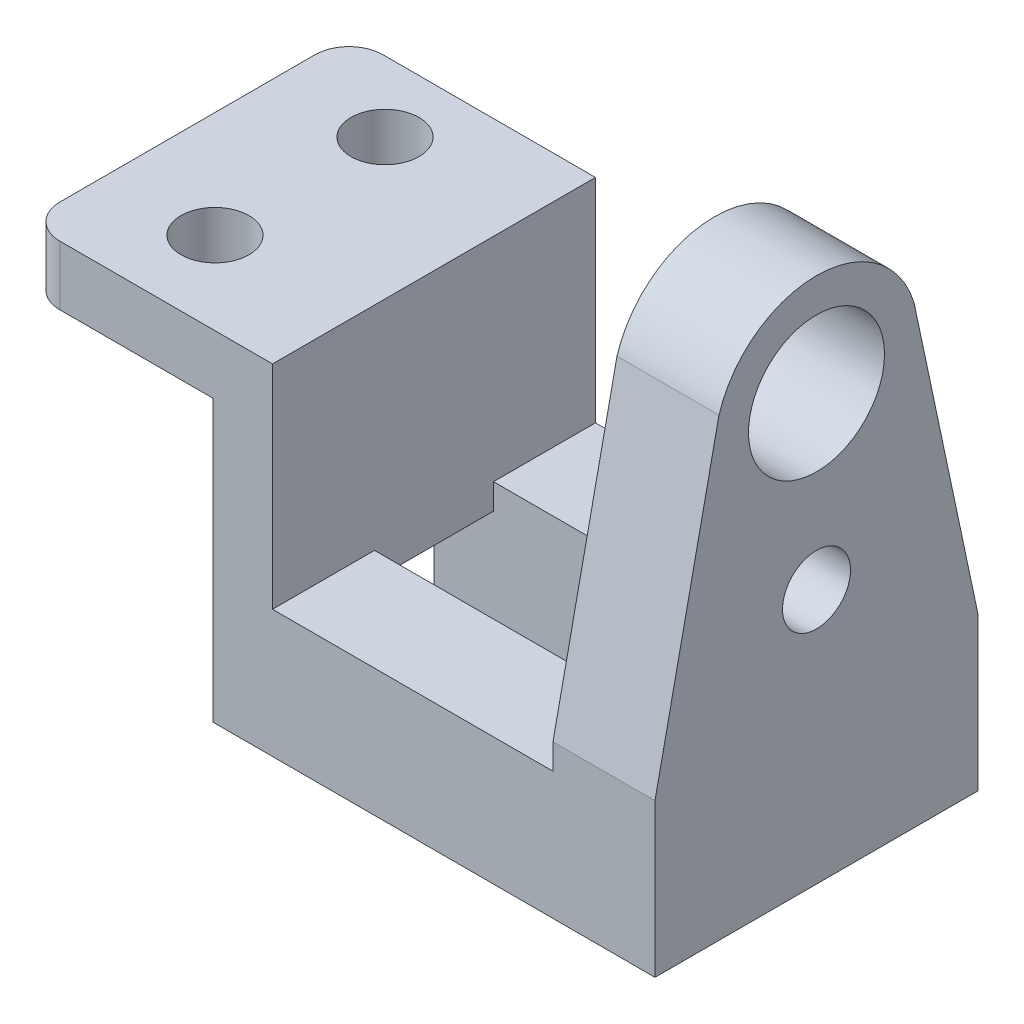
ISO-10303-21;
HEADER;
FILE_DESCRIPTION(('STEP AP214'),'2;1');
FILE_NAME('part.step','',(''),(''),'','','');
FILE_SCHEMA(('AUTOMOTIVE_DESIGN { 1 0 10303 214 1 1 1 1 }'));
ENDSEC;
DATA;
#1=APPLICATION_CONTEXT('core data for automotive mechanical design processes');
#2=APPLICATION_PROTOCOL_DEFINITION('international standard','automotive_design',2000,#1);
#3=PRODUCT_CONTEXT('',#1,'mechanical');
#4=PRODUCT('Part','Part','',(#3));
#5=PRODUCT_RELATED_PRODUCT_CATEGORY('part','',(#4));
#6=PRODUCT_DEFINITION_FORMATION('','',#4);
#7=PRODUCT_DEFINITION_CONTEXT('part definition',#1,'design');
#8=PRODUCT_DEFINITION('design','',#6,#7);
#9=PRODUCT_DEFINITION_SHAPE('','',#8);
#10=(LENGTH_UNIT() NAMED_UNIT(*) SI_UNIT(.MILLI.,.METRE.));
#11=(NAMED_UNIT(*) PLANE_ANGLE_UNIT() SI_UNIT($,.RADIAN.));
#12=(NAMED_UNIT(*) SI_UNIT($,.STERADIAN.) SOLID_ANGLE_UNIT());
#13=UNCERTAINTY_MEASURE_WITH_UNIT(LENGTH_MEASURE(1.E-05),#10,'distance_accuracy_value','');
#14=(GEOMETRIC_REPRESENTATION_CONTEXT(3) GLOBAL_UNCERTAINTY_ASSIGNED_CONTEXT((#13)) GLOBAL_UNIT_ASSIGNED_CONTEXT((#10,
#11,#12)) REPRESENTATION_CONTEXT('',''));
#15=CARTESIAN_POINT('',(0.,0.,0.));
#16=DIRECTION('',(0.,0.,1.));
#17=DIRECTION('',(1.,0.,0.));
#18=AXIS2_PLACEMENT_3D('',#15,#16,#17);
#19=CARTESIAN_POINT('',(7.,8.,38.));
#20=DIRECTION('',(-1.,0.,0.));
#21=DIRECTION('',(0.,0.,1.));
#22=AXIS2_PLACEMENT_3D('',#19,#20,#21);
#23=PLANE('',#22);
#24=DIRECTION('',(0.,-1.,0.));
#25=VECTOR('',#24,1.);
#26=CARTESIAN_POINT('',(7.,15.,12.));
#27=LINE('',#26,#25);
#28=CARTESIAN_POINT('',(7.,15.,12.));
#29=VERTEX_POINT('',#28);
#30=CARTESIAN_POINT('',(6.99999999999998,12.,12.));
#31=VERTEX_POINT('',#30);
#32=EDGE_CURVE('E58',#29,#31,#27,.T.);
#33=ORIENTED_EDGE('',*,*,#32,.F.);
#34=DIRECTION('',(0.,0.,1.));
#35=VECTOR('',#34,1.);
#36=CARTESIAN_POINT('',(7.,15.,12.));
#37=LINE('',#36,#35);
#38=CARTESIAN_POINT('',(7.,15.,0.));
#39=VERTEX_POINT('',#38);
#40=EDGE_CURVE('E406',#39,#29,#37,.T.);
#41=ORIENTED_EDGE('',*,*,#40,.F.);
#42=DIRECTION('',(0.,1.,0.));
#43=VECTOR('',#42,1.);
#44=CARTESIAN_POINT('',(7.,8.,0.));
#45=LINE('',#44,#43);
#46=CARTESIAN_POINT('',(7.,40.,0.));
#47=VERTEX_POINT('',#46);
#48=EDGE_CURVE('E292',#39,#47,#45,.T.);
#49=ORIENTED_EDGE('',*,*,#48,.T.);
#50=DIRECTION('',(0.,0.,1.));
#51=VECTOR('',#50,1.);
#52=CARTESIAN_POINT('',(7.,40.,0.));
#53=LINE('',#52,#51);
#54=CARTESIAN_POINT('',(7.,40.,38.));
#55=VERTEX_POINT('',#54);
#56=EDGE_CURVE('E236',#47,#55,#53,.T.);
#57=ORIENTED_EDGE('',*,*,#56,.T.);
#58=DIRECTION('',(0.,1.,0.));
#59=VECTOR('',#58,1.);
#60=CARTESIAN_POINT('',(7.,8.,38.));
#61=LINE('',#60,#59);
#62=CARTESIAN_POINT('',(7.,15.,38.));
#63=VERTEX_POINT('',#62);
#64=EDGE_CURVE('E301',#63,#55,#61,.T.);
#65=ORIENTED_EDGE('',*,*,#64,.F.);
#66=DIRECTION('',(0.,0.,1.));
#67=VECTOR('',#66,1.);
#68=CARTESIAN_POINT('',(7.,15.,38.));
#69=LINE('',#68,#67);
#70=CARTESIAN_POINT('',(7.,15.,26.));
#71=VERTEX_POINT('',#70);
#72=EDGE_CURVE('E349',#71,#63,#69,.T.);
#73=ORIENTED_EDGE('',*,*,#72,.F.);
#74=DIRECTION('',(0.,-1.,0.));
#75=VECTOR('',#74,1.);
#76=CARTESIAN_POINT('',(7.,15.,26.));
#77=LINE('',#76,#75);
#78=CARTESIAN_POINT('',(7.,12.,26.));
#79=VERTEX_POINT('',#78);
#80=EDGE_CURVE('E348',#71,#79,#77,.T.);
#81=ORIENTED_EDGE('',*,*,#80,.T.);
#82=DIRECTION('',(0.,0.,1.));
#83=VECTOR('',#82,1.);
#84=CARTESIAN_POINT('',(7.,12.,38.));
#85=LINE('',#84,#83);
#86=EDGE_CURVE('E11',#31,#79,#85,.T.);
#87=ORIENTED_EDGE('',*,*,#86,.F.);
#88=EDGE_LOOP('',(#33,#41,#49,#57,#65,#73,#81,#87));
#89=FACE_BOUND('',#88,.T.);
#90=ADVANCED_FACE('F44',(#89),#23,.F.);
#91=CARTESIAN_POINT('',(40.,18.,38.));
#92=DIRECTION('',(1.,0.,0.));
#93=DIRECTION('',(0.,0.,-1.));
#94=AXIS2_PLACEMENT_3D('',#91,#92,#93);
#95=PLANE('',#94);
#96=CARTESIAN_POINT('',(40.,30.,19.));
#97=DIRECTION('',(1.,0.,0.));
#98=DIRECTION('',(0.,0.,-1.));
#99=AXIS2_PLACEMENT_3D('',#96,#97,#98);
#100=CIRCLE('',#99,4.);
#101=CARTESIAN_POINT('',(40.,30.,15.));
#102=VERTEX_POINT('',#101);
#103=EDGE_CURVE('E357',#102,#102,#100,.T.);
#104=ORIENTED_EDGE('',*,*,#103,.T.);
#105=EDGE_LOOP('',(#104));
#106=FACE_BOUND('',#105,.T.);
#107=CARTESIAN_POINT('',(40.,50.,19.));
#108=DIRECTION('',(1.,0.,0.));
#109=DIRECTION('',(0.,0.,-1.));
#110=AXIS2_PLACEMENT_3D('',#107,#108,#109);
#111=CIRCLE('',#110,8.);
#112=CARTESIAN_POINT('',(40.,50.,11.));
#113=VERTEX_POINT('',#112);
#114=EDGE_CURVE('E366',#113,#113,#111,.T.);
#115=ORIENTED_EDGE('',*,*,#114,.T.);
#116=EDGE_LOOP('',(#115));
#117=FACE_BOUND('',#116,.T.);
#118=DIRECTION('',(0.,0.,-1.));
#119=VECTOR('',#118,1.);
#120=CARTESIAN_POINT('',(40.,15.,0.));
#121=LINE('',#120,#119);
#122=CARTESIAN_POINT('',(40.,15.,12.));
#123=VERTEX_POINT('',#122);
#124=CARTESIAN_POINT('',(40.,15.,0.));
#125=VERTEX_POINT('',#124);
#126=EDGE_CURVE('E410',#123,#125,#121,.T.);
#127=ORIENTED_EDGE('',*,*,#126,.F.);
#128=DIRECTION('',(0.,1.,0.));
#129=VECTOR('',#128,1.);
#130=CARTESIAN_POINT('',(40.,12.,12.));
#131=LINE('',#130,#129);
#132=CARTESIAN_POINT('',(40.,0.,12.));
#133=VERTEX_POINT('',#132);
#134=EDGE_CURVE('E70',#133,#123,#131,.T.);
#135=ORIENTED_EDGE('',*,*,#134,.F.);
#136=DIRECTION('',(0.,0.,-1.));
#137=VECTOR('',#136,1.);
#138=CARTESIAN_POINT('',(40.,0.,38.));
#139=LINE('',#138,#137);
#140=CARTESIAN_POINT('',(40.,0.,26.));
#141=VERTEX_POINT('',#140);
#142=EDGE_CURVE('E239',#141,#133,#139,.T.);
#143=ORIENTED_EDGE('',*,*,#142,.F.);
#144=DIRECTION('',(0.,-1.,0.));
#145=VECTOR('',#144,1.);
#146=CARTESIAN_POINT('',(40.,0.,26.));
#147=LINE('',#146,#145);
#148=CARTESIAN_POINT('',(40.,15.,26.));
#149=VERTEX_POINT('',#148);
#150=EDGE_CURVE('E241',#149,#141,#147,.T.);
#151=ORIENTED_EDGE('',*,*,#150,.F.);
#152=DIRECTION('',(0.,0.,-1.));
#153=VECTOR('',#152,1.);
#154=CARTESIAN_POINT('',(40.,15.,26.));
#155=LINE('',#154,#153);
#156=CARTESIAN_POINT('',(40.,15.,38.));
#157=VERTEX_POINT('',#156);
#158=EDGE_CURVE('E360',#157,#149,#155,.T.);
#159=ORIENTED_EDGE('',*,*,#158,.F.);
#160=DIRECTION('',(0.,-1.,0.));
#161=VECTOR('',#160,1.);
#162=CARTESIAN_POINT('',(40.,18.,38.));
#163=LINE('',#162,#161);
#164=CARTESIAN_POINT('',(40.,18.,38.));
#165=VERTEX_POINT('',#164);
#166=EDGE_CURVE('E296',#165,#157,#163,.T.);
#167=ORIENTED_EDGE('',*,*,#166,.F.);
#168=DIRECTION('',(0.,-0.978272196346445,0.207324648451413));
#169=VECTOR('',#168,1.);
#170=CARTESIAN_POINT('',(40.,18.,38.));
#171=LINE('',#170,#169);
#172=CARTESIAN_POINT('',(40.,53.5184745322787,30.4725906823919));
#173=VERTEX_POINT('',#172);
#174=EDGE_CURVE('E270',#173,#165,#171,.T.);
#175=ORIENTED_EDGE('',*,*,#174,.F.);
#176=CARTESIAN_POINT('',(40.,50.,19.));
#177=DIRECTION('',(1.,0.,0.));
#178=DIRECTION('',(0.,0.,-1.));
#179=AXIS2_PLACEMENT_3D('',#176,#177,#178);
#180=CIRCLE('',#179,12.);
#181=CARTESIAN_POINT('',(40.,53.5184745322787,7.52740931760806));
#182=VERTEX_POINT('',#181);
#183=EDGE_CURVE('E274',#182,#173,#180,.T.);
#184=ORIENTED_EDGE('',*,*,#183,.F.);
#185=DIRECTION('',(0.,0.978272196346445,0.207324648451413));
#186=VECTOR('',#185,1.);
#187=CARTESIAN_POINT('',(40.,18.,0.));
#188=LINE('',#187,#186);
#189=CARTESIAN_POINT('',(40.,18.,0.));
#190=VERTEX_POINT('',#189);
#191=EDGE_CURVE('E267',#190,#182,#188,.T.);
#192=ORIENTED_EDGE('',*,*,#191,.F.);
#193=DIRECTION('',(0.,-1.,0.));
#194=VECTOR('',#193,1.);
#195=CARTESIAN_POINT('',(40.,18.,0.));
#196=LINE('',#195,#194);
#197=EDGE_CURVE('E315',#190,#125,#196,.T.);
#198=ORIENTED_EDGE('',*,*,#197,.T.);
#199=EDGE_LOOP('',(#127,#135,#143,#151,#159,#167,#175,#184,#192,#198));
#200=FACE_BOUND('',#199,.T.);
#201=ADVANCED_FACE('F421',(#106,#117,#200),#95,.F.);
#202=CARTESIAN_POINT('',(0.,0.,38.));
#203=DIRECTION('',(1.,0.,0.));
#204=DIRECTION('',(0.,0.,-1.));
#205=AXIS2_PLACEMENT_3D('',#202,#203,#204);
#206=PLANE('',#205);
#207=DIRECTION('',(0.,-1.,0.));
#208=VECTOR('',#207,1.);
#209=CARTESIAN_POINT('',(0.,0.,38.));
#210=LINE('',#209,#208);
#211=CARTESIAN_POINT('',(0.,33.,38.));
#212=VERTEX_POINT('',#211);
#213=CARTESIAN_POINT('',(0.,0.,38.));
#214=VERTEX_POINT('',#213);
#215=EDGE_CURVE('E289',#212,#214,#210,.T.);
#216=ORIENTED_EDGE('',*,*,#215,.F.);
#217=DIRECTION('',(0.,0.,-1.));
#218=VECTOR('',#217,1.);
#219=CARTESIAN_POINT('',(0.,33.,0.));
#220=LINE('',#219,#218);
#221=CARTESIAN_POINT('',(0.,33.,0.));
#222=VERTEX_POINT('',#221);
#223=EDGE_CURVE('E219',#212,#222,#220,.T.);
#224=ORIENTED_EDGE('',*,*,#223,.T.);
#225=DIRECTION('',(0.,-1.,0.));
#226=VECTOR('',#225,1.);
#227=CARTESIAN_POINT('',(0.,0.,0.));
#228=LINE('',#227,#226);
#229=CARTESIAN_POINT('',(0.,0.,0.));
#230=VERTEX_POINT('',#229);
#231=EDGE_CURVE('E290',#222,#230,#228,.T.);
#232=ORIENTED_EDGE('',*,*,#231,.T.);
#233=DIRECTION('',(0.,0.,-1.));
#234=VECTOR('',#233,1.);
#235=CARTESIAN_POINT('',(0.,0.,38.));
#236=LINE('',#235,#234);
#237=CARTESIAN_POINT('',(0.,0.,12.));
#238=VERTEX_POINT('',#237);
#239=EDGE_CURVE('E317',#238,#230,#236,.T.);
#240=ORIENTED_EDGE('',*,*,#239,.F.);
#241=DIRECTION('',(0.,1.,0.));
#242=VECTOR('',#241,1.);
#243=CARTESIAN_POINT('',(0.,12.,12.));
#244=LINE('',#243,#242);
#245=CARTESIAN_POINT('',(0.,12.,12.));
#246=VERTEX_POINT('',#245);
#247=EDGE_CURVE('E244',#238,#246,#244,.T.);
#248=ORIENTED_EDGE('',*,*,#247,.T.);
#249=DIRECTION('',(0.,0.,1.));
#250=VECTOR('',#249,1.);
#251=CARTESIAN_POINT('',(0.,12.,26.));
#252=LINE('',#251,#250);
#253=CARTESIAN_POINT('',(0.,12.,26.));
#254=VERTEX_POINT('',#253);
#255=EDGE_CURVE('E248',#246,#254,#252,.T.);
#256=ORIENTED_EDGE('',*,*,#255,.T.);
#257=DIRECTION('',(0.,-1.,0.));
#258=VECTOR('',#257,1.);
#259=CARTESIAN_POINT('',(0.,0.,26.));
#260=LINE('',#259,#258);
#261=CARTESIAN_POINT('',(0.,0.,26.));
#262=VERTEX_POINT('',#261);
#263=EDGE_CURVE('E246',#254,#262,#260,.T.);
#264=ORIENTED_EDGE('',*,*,#263,.T.);
#265=EDGE_CURVE('E52',#214,#262,#236,.T.);
#266=ORIENTED_EDGE('',*,*,#265,.F.);
#267=EDGE_LOOP('',(#216,#224,#232,#240,#248,#256,#264,#266));
#268=FACE_BOUND('',#267,.T.);
#269=ADVANCED_FACE('F50',(#268),#206,.F.);
#270=CARTESIAN_POINT('',(0.,0.,38.));
#271=DIRECTION('',(0.,1.,0.));
#272=DIRECTION('',(0.,0.,1.));
#273=AXIS2_PLACEMENT_3D('',#270,#271,#272);
#274=PLANE('',#273);
#275=DIRECTION('',(1.,0.,0.));
#276=VECTOR('',#275,1.);
#277=CARTESIAN_POINT('',(-111.747483193135,0.,26.));
#278=LINE('',#277,#276);
#279=EDGE_CURVE('E261',#262,#141,#278,.T.);
#280=ORIENTED_EDGE('',*,*,#279,.T.);
#281=ORIENTED_EDGE('',*,*,#142,.T.);
#282=DIRECTION('',(1.,0.,0.));
#283=VECTOR('',#282,1.);
#284=CARTESIAN_POINT('',(-111.747483193135,0.,12.));
#285=LINE('',#284,#283);
#286=EDGE_CURVE('E243',#238,#133,#285,.T.);
#287=ORIENTED_EDGE('',*,*,#286,.F.);
#288=ORIENTED_EDGE('',*,*,#239,.T.);
#289=DIRECTION('',(1.,0.,0.));
#290=VECTOR('',#289,1.);
#291=CARTESIAN_POINT('',(0.,0.,0.));
#292=LINE('',#291,#290);
#293=CARTESIAN_POINT('',(52.,0.,0.));
#294=VERTEX_POINT('',#293);
#295=EDGE_CURVE('E304',#230,#294,#292,.T.);
#296=ORIENTED_EDGE('',*,*,#295,.T.);
#297=DIRECTION('',(0.,0.,-1.));
#298=VECTOR('',#297,1.);
#299=CARTESIAN_POINT('',(52.,0.,38.));
#300=LINE('',#299,#298);
#301=CARTESIAN_POINT('',(52.,0.,38.));
#302=VERTEX_POINT('',#301);
#303=EDGE_CURVE('E303',#302,#294,#300,.T.);
#304=ORIENTED_EDGE('',*,*,#303,.F.);
#305=DIRECTION('',(1.,0.,0.));
#306=VECTOR('',#305,1.);
#307=CARTESIAN_POINT('',(0.,0.,38.));
#308=LINE('',#307,#306);
#309=EDGE_CURVE('E293',#214,#302,#308,.T.);
#310=ORIENTED_EDGE('',*,*,#309,.F.);
#311=ORIENTED_EDGE('',*,*,#265,.T.);
#312=EDGE_LOOP('',(#280,#281,#287,#288,#296,#304,#310,#311));
#313=FACE_BOUND('',#312,.T.);
#314=ADVANCED_FACE('F324',(#313),#274,.F.);
#315=CARTESIAN_POINT('',(52.,0.,38.));
#316=DIRECTION('',(-1.,0.,0.));
#317=DIRECTION('',(0.,0.,1.));
#318=AXIS2_PLACEMENT_3D('',#315,#316,#317);
#319=PLANE('',#318);
#320=CARTESIAN_POINT('',(52.,30.,19.));
#321=DIRECTION('',(1.,0.,0.));
#322=DIRECTION('',(0.,0.,-1.));
#323=AXIS2_PLACEMENT_3D('',#320,#321,#322);
#324=CIRCLE('',#323,4.);
#325=CARTESIAN_POINT('',(52.,30.,15.));
#326=VERTEX_POINT('',#325);
#327=EDGE_CURVE('E351',#326,#326,#324,.T.);
#328=ORIENTED_EDGE('',*,*,#327,.F.);
#329=EDGE_LOOP('',(#328));
#330=FACE_BOUND('',#329,.T.);
#331=CARTESIAN_POINT('',(52.,50.,19.));
#332=DIRECTION('',(1.,0.,0.));
#333=DIRECTION('',(0.,0.,-1.));
#334=AXIS2_PLACEMENT_3D('',#331,#332,#333);
#335=CIRCLE('',#334,8.);
#336=CARTESIAN_POINT('',(52.,50.,11.));
#337=VERTEX_POINT('',#336);
#338=EDGE_CURVE('E364',#337,#337,#335,.T.);
#339=ORIENTED_EDGE('',*,*,#338,.F.);
#340=EDGE_LOOP('',(#339));
#341=FACE_BOUND('',#340,.T.);
#342=DIRECTION('',(0.,1.,0.));
#343=VECTOR('',#342,1.);
#344=CARTESIAN_POINT('',(52.,0.,0.));
#345=LINE('',#344,#343);
#346=CARTESIAN_POINT('',(52.,18.,0.));
#347=VERTEX_POINT('',#346);
#348=EDGE_CURVE('E310',#294,#347,#345,.T.);
#349=ORIENTED_EDGE('',*,*,#348,.T.);
#350=DIRECTION('',(0.,0.978272196346445,0.207324648451413));
#351=VECTOR('',#350,1.);
#352=CARTESIAN_POINT('',(52.,18.,0.));
#353=LINE('',#352,#351);
#354=CARTESIAN_POINT('',(52.,53.5184745322787,7.52740931760806));
#355=VERTEX_POINT('',#354);
#356=EDGE_CURVE('E279',#347,#355,#353,.T.);
#357=ORIENTED_EDGE('',*,*,#356,.T.);
#358=CARTESIAN_POINT('',(52.,50.,19.));
#359=DIRECTION('',(1.,0.,0.));
#360=DIRECTION('',(0.,0.,-1.));
#361=AXIS2_PLACEMENT_3D('',#358,#359,#360);
#362=CIRCLE('',#361,12.);
#363=CARTESIAN_POINT('',(52.,53.5184745322787,30.4725906823919));
#364=VERTEX_POINT('',#363);
#365=EDGE_CURVE('E272',#355,#364,#362,.T.);
#366=ORIENTED_EDGE('',*,*,#365,.T.);
#367=DIRECTION('',(0.,-0.978272196346445,0.207324648451413));
#368=VECTOR('',#367,1.);
#369=CARTESIAN_POINT('',(52.,18.,38.));
#370=LINE('',#369,#368);
#371=CARTESIAN_POINT('',(52.,18.,38.));
#372=VERTEX_POINT('',#371);
#373=EDGE_CURVE('E262',#364,#372,#370,.T.);
#374=ORIENTED_EDGE('',*,*,#373,.T.);
#375=DIRECTION('',(0.,1.,0.));
#376=VECTOR('',#375,1.);
#377=CARTESIAN_POINT('',(52.,0.,38.));
#378=LINE('',#377,#376);
#379=EDGE_CURVE('E295',#302,#372,#378,.T.);
#380=ORIENTED_EDGE('',*,*,#379,.F.);
#381=ORIENTED_EDGE('',*,*,#303,.T.);
#382=EDGE_LOOP('',(#349,#357,#366,#374,#380,#381));
#383=FACE_BOUND('',#382,.T.);
#384=ADVANCED_FACE('F337',(#330,#341,#383),#319,.F.);
#385=CARTESIAN_POINT('',(0.,0.,38.));
#386=DIRECTION('',(0.,0.,1.));
#387=DIRECTION('',(1.,0.,0.));
#388=AXIS2_PLACEMENT_3D('',#385,#386,#387);
#389=PLANE('',#388);
#390=DIRECTION('',(1.,0.,0.));
#391=VECTOR('',#390,1.);
#392=CARTESIAN_POINT('',(40.,15.,38.));
#393=LINE('',#392,#391);
#394=EDGE_CURVE('E414',#63,#157,#393,.T.);
#395=ORIENTED_EDGE('',*,*,#394,.F.);
#396=ORIENTED_EDGE('',*,*,#64,.T.);
#397=DIRECTION('',(-1.,0.,0.));
#398=VECTOR('',#397,1.);
#399=CARTESIAN_POINT('',(7.,40.,38.));
#400=LINE('',#399,#398);
#401=CARTESIAN_POINT('',(-18.,40.,38.));
#402=VERTEX_POINT('',#401);
#403=EDGE_CURVE('E230',#55,#402,#400,.T.);
#404=ORIENTED_EDGE('',*,*,#403,.T.);
#405=DIRECTION('',(0.,1.,0.));
#406=VECTOR('',#405,1.);
#407=CARTESIAN_POINT('',(-18.,33.,38.));
#408=LINE('',#407,#406);
#409=CARTESIAN_POINT('',(-18.,33.,38.));
#410=VERTEX_POINT('',#409);
#411=EDGE_CURVE('E229',#410,#402,#408,.T.);
#412=ORIENTED_EDGE('',*,*,#411,.F.);
#413=DIRECTION('',(1.,0.,0.));
#414=VECTOR('',#413,1.);
#415=CARTESIAN_POINT('',(-18.,33.,38.));
#416=LINE('',#415,#414);
#417=EDGE_CURVE('E220',#410,#212,#416,.T.);
#418=ORIENTED_EDGE('',*,*,#417,.T.);
#419=ORIENTED_EDGE('',*,*,#215,.T.);
#420=ORIENTED_EDGE('',*,*,#309,.T.);
#421=ORIENTED_EDGE('',*,*,#379,.T.);
#422=DIRECTION('',(-1.,0.,0.));
#423=VECTOR('',#422,1.);
#424=CARTESIAN_POINT('',(52.,18.,38.));
#425=LINE('',#424,#423);
#426=EDGE_CURVE('E298',#372,#165,#425,.T.);
#427=ORIENTED_EDGE('',*,*,#426,.T.);
#428=ORIENTED_EDGE('',*,*,#166,.T.);
#429=EDGE_LOOP('',(#395,#396,#404,#412,#418,#419,#420,#421,#427,#428));
#430=FACE_BOUND('',#429,.T.);
#431=ADVANCED_FACE('F394',(#430),#389,.T.);
#432=CARTESIAN_POINT('',(0.,0.,0.));
#433=DIRECTION('',(0.,0.,1.));
#434=DIRECTION('',(1.,0.,0.));
#435=AXIS2_PLACEMENT_3D('',#432,#433,#434);
#436=PLANE('',#435);
#437=ORIENTED_EDGE('',*,*,#48,.F.);
#438=DIRECTION('',(-1.,0.,0.));
#439=VECTOR('',#438,1.);
#440=CARTESIAN_POINT('',(7.,15.,0.));
#441=LINE('',#440,#439);
#442=EDGE_CURVE('E397',#125,#39,#441,.T.);
#443=ORIENTED_EDGE('',*,*,#442,.F.);
#444=ORIENTED_EDGE('',*,*,#197,.F.);
#445=DIRECTION('',(-1.,0.,0.));
#446=VECTOR('',#445,1.);
#447=CARTESIAN_POINT('',(52.,18.,0.));
#448=LINE('',#447,#446);
#449=EDGE_CURVE('E307',#347,#190,#448,.T.);
#450=ORIENTED_EDGE('',*,*,#449,.F.);
#451=ORIENTED_EDGE('',*,*,#348,.F.);
#452=ORIENTED_EDGE('',*,*,#295,.F.);
#453=ORIENTED_EDGE('',*,*,#231,.F.);
#454=DIRECTION('',(-1.,0.,0.));
#455=VECTOR('',#454,1.);
#456=CARTESIAN_POINT('',(0.,33.,0.));
#457=LINE('',#456,#455);
#458=CARTESIAN_POINT('',(-18.,33.,0.));
#459=VERTEX_POINT('',#458);
#460=EDGE_CURVE('E192',#222,#459,#457,.T.);
#461=ORIENTED_EDGE('',*,*,#460,.T.);
#462=DIRECTION('',(0.,1.,0.));
#463=VECTOR('',#462,1.);
#464=CARTESIAN_POINT('',(-18.,33.,0.));
#465=LINE('',#464,#463);
#466=CARTESIAN_POINT('',(-18.,40.,0.));
#467=VERTEX_POINT('',#466);
#468=EDGE_CURVE('E210',#459,#467,#465,.T.);
#469=ORIENTED_EDGE('',*,*,#468,.T.);
#470=DIRECTION('',(-1.,0.,0.));
#471=VECTOR('',#470,1.);
#472=CARTESIAN_POINT('',(7.,40.,0.));
#473=LINE('',#472,#471);
#474=EDGE_CURVE('E234',#47,#467,#473,.T.);
#475=ORIENTED_EDGE('',*,*,#474,.F.);
#476=EDGE_LOOP('',(#437,#443,#444,#450,#451,#452,#453,#461,#469,#475));
#477=FACE_BOUND('',#476,.T.);
#478=ADVANCED_FACE('F335',(#477),#436,.F.);
#479=CARTESIAN_POINT('',(40.,18.,38.));
#480=DIRECTION('',(0.,0.207324648451413,0.978272196346445));
#481=DIRECTION('',(0.,-0.978272196346445,0.207324648451413));
#482=AXIS2_PLACEMENT_3D('',#479,#480,#481);
#483=PLANE('',#482);
#484=ORIENTED_EDGE('',*,*,#373,.F.);
#485=DIRECTION('',(1.,0.,0.));
#486=VECTOR('',#485,1.);
#487=CARTESIAN_POINT('',(40.,53.5184745322787,30.4725906823919));
#488=LINE('',#487,#486);
#489=EDGE_CURVE('E284',#173,#364,#488,.T.);
#490=ORIENTED_EDGE('',*,*,#489,.F.);
#491=ORIENTED_EDGE('',*,*,#174,.T.);
#492=ORIENTED_EDGE('',*,*,#426,.F.);
#493=EDGE_LOOP('',(#484,#490,#491,#492));
#494=FACE_BOUND('',#493,.T.);
#495=ADVANCED_FACE('F611',(#494),#483,.T.);
#496=CARTESIAN_POINT('',(40.,50.,19.));
#497=DIRECTION('',(1.,0.,0.));
#498=DIRECTION('',(0.,0.,-1.));
#499=AXIS2_PLACEMENT_3D('',#496,#497,#498);
#500=CYLINDRICAL_SURFACE('',#499,12.);
#501=ORIENTED_EDGE('',*,*,#365,.F.);
#502=DIRECTION('',(1.,0.,0.));
#503=VECTOR('',#502,1.);
#504=CARTESIAN_POINT('',(40.,53.5184745322787,7.52740931760806));
#505=LINE('',#504,#503);
#506=EDGE_CURVE('E280',#182,#355,#505,.T.);
#507=ORIENTED_EDGE('',*,*,#506,.F.);
#508=ORIENTED_EDGE('',*,*,#183,.T.);
#509=ORIENTED_EDGE('',*,*,#489,.T.);
#510=EDGE_LOOP('',(#501,#507,#508,#509));
#511=FACE_BOUND('',#510,.T.);
#512=ADVANCED_FACE('F675',(#511),#500,.T.);
#513=CARTESIAN_POINT('',(40.,18.,0.));
#514=DIRECTION('',(0.,0.207324648451413,-0.978272196346445));
#515=DIRECTION('',(0.,0.978272196346445,0.207324648451413));
#516=AXIS2_PLACEMENT_3D('',#513,#514,#515);
#517=PLANE('',#516);
#518=ORIENTED_EDGE('',*,*,#356,.F.);
#519=ORIENTED_EDGE('',*,*,#449,.T.);
#520=ORIENTED_EDGE('',*,*,#191,.T.);
#521=ORIENTED_EDGE('',*,*,#506,.T.);
#522=EDGE_LOOP('',(#518,#519,#520,#521));
#523=FACE_BOUND('',#522,.T.);
#524=ADVANCED_FACE('F568',(#523),#517,.T.);
#525=CARTESIAN_POINT('',(-111.747483193135,0.,26.));
#526=DIRECTION('',(0.,0.,-1.));
#527=DIRECTION('',(-1.,0.,0.));
#528=AXIS2_PLACEMENT_3D('',#525,#526,#527);
#529=PLANE('',#528);
#530=DIRECTION('',(1.,0.,0.));
#531=VECTOR('',#530,1.);
#532=CARTESIAN_POINT('',(-111.747483193135,12.,26.));
#533=LINE('',#532,#531);
#534=EDGE_CURVE('E257',#254,#79,#533,.T.);
#535=ORIENTED_EDGE('',*,*,#534,.T.);
#536=ORIENTED_EDGE('',*,*,#80,.F.);
#537=DIRECTION('',(-1.,0.,0.));
#538=VECTOR('',#537,1.);
#539=CARTESIAN_POINT('',(7.,15.,26.));
#540=LINE('',#539,#538);
#541=EDGE_CURVE('E354',#149,#71,#540,.T.);
#542=ORIENTED_EDGE('',*,*,#541,.F.);
#543=ORIENTED_EDGE('',*,*,#150,.T.);
#544=ORIENTED_EDGE('',*,*,#279,.F.);
#545=ORIENTED_EDGE('',*,*,#263,.F.);
#546=EDGE_LOOP('',(#535,#536,#542,#543,#544,#545));
#547=FACE_BOUND('',#546,.T.);
#548=ADVANCED_FACE('F342',(#547),#529,.T.);
#549=CARTESIAN_POINT('',(-111.747483193135,12.,26.));
#550=DIRECTION('',(0.,-1.,0.));
#551=DIRECTION('',(0.,0.,-1.));
#552=AXIS2_PLACEMENT_3D('',#549,#550,#551);
#553=PLANE('',#552);
#554=DIRECTION('',(1.,0.,0.));
#555=VECTOR('',#554,1.);
#556=CARTESIAN_POINT('',(-111.747483193135,12.,12.));
#557=LINE('',#556,#555);
#558=EDGE_CURVE('E253',#246,#31,#557,.T.);
#559=ORIENTED_EDGE('',*,*,#558,.T.);
#560=ORIENTED_EDGE('',*,*,#86,.T.);
#561=ORIENTED_EDGE('',*,*,#534,.F.);
#562=ORIENTED_EDGE('',*,*,#255,.F.);
#563=EDGE_LOOP('',(#559,#560,#561,#562));
#564=FACE_BOUND('',#563,.T.);
#565=ADVANCED_FACE('F346',(#564),#553,.T.);
#566=CARTESIAN_POINT('',(-111.747483193135,12.,12.));
#567=DIRECTION('',(0.,0.,1.));
#568=DIRECTION('',(1.,0.,0.));
#569=AXIS2_PLACEMENT_3D('',#566,#567,#568);
#570=PLANE('',#569);
#571=ORIENTED_EDGE('',*,*,#32,.T.);
#572=ORIENTED_EDGE('',*,*,#558,.F.);
#573=ORIENTED_EDGE('',*,*,#247,.F.);
#574=ORIENTED_EDGE('',*,*,#286,.T.);
#575=ORIENTED_EDGE('',*,*,#134,.T.);
#576=DIRECTION('',(1.,0.,0.));
#577=VECTOR('',#576,1.);
#578=CARTESIAN_POINT('',(40.,15.,12.));
#579=LINE('',#578,#577);
#580=EDGE_CURVE('E409',#29,#123,#579,.T.);
#581=ORIENTED_EDGE('',*,*,#580,.F.);
#582=EDGE_LOOP('',(#571,#572,#573,#574,#575,#581));
#583=FACE_BOUND('',#582,.T.);
#584=ADVANCED_FACE('F390',(#583),#570,.T.);
#585=CARTESIAN_POINT('',(7.,40.,0.));
#586=DIRECTION('',(0.,1.,0.));
#587=DIRECTION('',(0.,0.,1.));
#588=AXIS2_PLACEMENT_3D('',#585,#586,#587);
#589=PLANE('',#588);
#590=CARTESIAN_POINT('',(-9.5,40.,8.26651502922683));
#591=DIRECTION('',(0.,1.,0.));
#592=DIRECTION('',(0.,0.,1.));
#593=AXIS2_PLACEMENT_3D('',#590,#591,#592);
#594=CIRCLE('',#593,4.);
#595=CARTESIAN_POINT('',(-9.5,40.,12.2665150292268));
#596=VERTEX_POINT('',#595);
#597=EDGE_CURVE('E373',#596,#596,#594,.T.);
#598=ORIENTED_EDGE('',*,*,#597,.F.);
#599=EDGE_LOOP('',(#598));
#600=FACE_BOUND('',#599,.T.);
#601=CARTESIAN_POINT('',(-9.5,40.,28.2665150292268));
#602=DIRECTION('',(0.,1.,0.));
#603=DIRECTION('',(0.,0.,1.));
#604=AXIS2_PLACEMENT_3D('',#601,#602,#603);
#605=CIRCLE('',#604,4.);
#606=CARTESIAN_POINT('',(-9.5,40.,32.2665150292268));
#607=VERTEX_POINT('',#606);
#608=EDGE_CURVE('E212',#607,#607,#605,.T.);
#609=ORIENTED_EDGE('',*,*,#608,.F.);
#610=EDGE_LOOP('',(#609));
#611=FACE_BOUND('',#610,.T.);
#612=ORIENTED_EDGE('',*,*,#403,.F.);
#613=ORIENTED_EDGE('',*,*,#56,.F.);
#614=ORIENTED_EDGE('',*,*,#474,.T.);
#615=CARTESIAN_POINT('',(-18.,40.,4.));
#616=DIRECTION('',(0.,1.,0.));
#617=DIRECTION('',(0.,0.,1.));
#618=AXIS2_PLACEMENT_3D('',#615,#616,#617);
#619=CIRCLE('',#618,4.);
#620=CARTESIAN_POINT('',(-22.,40.,4.));
#621=VERTEX_POINT('',#620);
#622=EDGE_CURVE('E224',#467,#621,#619,.T.);
#623=ORIENTED_EDGE('',*,*,#622,.T.);
#624=DIRECTION('',(0.,0.,1.));
#625=VECTOR('',#624,1.);
#626=CARTESIAN_POINT('',(-22.,40.,4.));
#627=LINE('',#626,#625);
#628=CARTESIAN_POINT('',(-22.,40.,34.));
#629=VERTEX_POINT('',#628);
#630=EDGE_CURVE('E190',#621,#629,#627,.T.);
#631=ORIENTED_EDGE('',*,*,#630,.T.);
#632=CARTESIAN_POINT('',(-18.,40.,34.));
#633=DIRECTION('',(0.,1.,0.));
#634=DIRECTION('',(0.,0.,1.));
#635=AXIS2_PLACEMENT_3D('',#632,#633,#634);
#636=CIRCLE('',#635,4.);
#637=EDGE_CURVE('E206',#629,#402,#636,.T.);
#638=ORIENTED_EDGE('',*,*,#637,.T.);
#639=EDGE_LOOP('',(#612,#613,#614,#623,#631,#638));
#640=FACE_BOUND('',#639,.T.);
#641=ADVANCED_FACE('F381',(#600,#611,#640),#589,.T.);
#642=CARTESIAN_POINT('',(-18.,33.,4.));
#643=DIRECTION('',(0.,1.,0.));
#644=DIRECTION('',(0.,0.,1.));
#645=AXIS2_PLACEMENT_3D('',#642,#643,#644);
#646=CYLINDRICAL_SURFACE('',#645,4.);
#647=ORIENTED_EDGE('',*,*,#622,.F.);
#648=ORIENTED_EDGE('',*,*,#468,.F.);
#649=CARTESIAN_POINT('',(-18.,33.,4.));
#650=DIRECTION('',(0.,1.,0.));
#651=DIRECTION('',(0.,0.,1.));
#652=AXIS2_PLACEMENT_3D('',#649,#650,#651);
#653=CIRCLE('',#652,4.);
#654=CARTESIAN_POINT('',(-22.,33.,4.));
#655=VERTEX_POINT('',#654);
#656=EDGE_CURVE('E197',#459,#655,#653,.T.);
#657=ORIENTED_EDGE('',*,*,#656,.T.);
#658=DIRECTION('',(0.,1.,0.));
#659=VECTOR('',#658,1.);
#660=CARTESIAN_POINT('',(-22.,33.,4.));
#661=LINE('',#660,#659);
#662=EDGE_CURVE('E185',#655,#621,#661,.T.);
#663=ORIENTED_EDGE('',*,*,#662,.T.);
#664=EDGE_LOOP('',(#647,#648,#657,#663));
#665=FACE_BOUND('',#664,.T.);
#666=ADVANCED_FACE('F202',(#665),#646,.T.);
#667=CARTESIAN_POINT('',(-18.,33.,34.));
#668=DIRECTION('',(0.,1.,0.));
#669=DIRECTION('',(0.,0.,1.));
#670=AXIS2_PLACEMENT_3D('',#667,#668,#669);
#671=CYLINDRICAL_SURFACE('',#670,4.);
#672=ORIENTED_EDGE('',*,*,#637,.F.);
#673=DIRECTION('',(0.,1.,0.));
#674=VECTOR('',#673,1.);
#675=CARTESIAN_POINT('',(-22.,33.,34.));
#676=LINE('',#675,#674);
#677=CARTESIAN_POINT('',(-22.,33.,34.));
#678=VERTEX_POINT('',#677);
#679=EDGE_CURVE('E195',#678,#629,#676,.T.);
#680=ORIENTED_EDGE('',*,*,#679,.F.);
#681=CARTESIAN_POINT('',(-18.,33.,34.));
#682=DIRECTION('',(0.,1.,0.));
#683=DIRECTION('',(0.,0.,1.));
#684=AXIS2_PLACEMENT_3D('',#681,#682,#683);
#685=CIRCLE('',#684,4.);
#686=EDGE_CURVE('E201',#678,#410,#685,.T.);
#687=ORIENTED_EDGE('',*,*,#686,.T.);
#688=ORIENTED_EDGE('',*,*,#411,.T.);
#689=EDGE_LOOP('',(#672,#680,#687,#688));
#690=FACE_BOUND('',#689,.T.);
#691=ADVANCED_FACE('F400',(#690),#671,.T.);
#692=CARTESIAN_POINT('',(-22.,33.,4.));
#693=DIRECTION('',(-1.,0.,0.));
#694=DIRECTION('',(0.,0.,1.));
#695=AXIS2_PLACEMENT_3D('',#692,#693,#694);
#696=PLANE('',#695);
#697=ORIENTED_EDGE('',*,*,#630,.F.);
#698=ORIENTED_EDGE('',*,*,#662,.F.);
#699=DIRECTION('',(0.,0.,1.));
#700=VECTOR('',#699,1.);
#701=CARTESIAN_POINT('',(-22.,33.,4.));
#702=LINE('',#701,#700);
#703=EDGE_CURVE('E184',#655,#678,#702,.T.);
#704=ORIENTED_EDGE('',*,*,#703,.T.);
#705=ORIENTED_EDGE('',*,*,#679,.T.);
#706=EDGE_LOOP('',(#697,#698,#704,#705));
#707=FACE_BOUND('',#706,.T.);
#708=ADVANCED_FACE('F183',(#707),#696,.T.);
#709=CARTESIAN_POINT('',(-18.,33.,4.));
#710=DIRECTION('',(0.,1.,0.));
#711=DIRECTION('',(0.,0.,1.));
#712=AXIS2_PLACEMENT_3D('',#709,#710,#711);
#713=PLANE('',#712);
#714=CARTESIAN_POINT('',(-9.5,33.,8.26651502922683));
#715=DIRECTION('',(0.,1.,0.));
#716=DIRECTION('',(0.,0.,1.));
#717=AXIS2_PLACEMENT_3D('',#714,#715,#716);
#718=CIRCLE('',#717,4.);
#719=CARTESIAN_POINT('',(-9.5,33.,12.2665150292268));
#720=VERTEX_POINT('',#719);
#721=EDGE_CURVE('E228',#720,#720,#718,.T.);
#722=ORIENTED_EDGE('',*,*,#721,.T.);
#723=EDGE_LOOP('',(#722));
#724=FACE_BOUND('',#723,.T.);
#725=CARTESIAN_POINT('',(-9.5,33.,28.2665150292268));
#726=DIRECTION('',(0.,1.,0.));
#727=DIRECTION('',(0.,0.,1.));
#728=AXIS2_PLACEMENT_3D('',#725,#726,#727);
#729=CIRCLE('',#728,4.);
#730=CARTESIAN_POINT('',(-9.5,33.,32.2665150292268));
#731=VERTEX_POINT('',#730);
#732=EDGE_CURVE('E374',#731,#731,#729,.T.);
#733=ORIENTED_EDGE('',*,*,#732,.T.);
#734=EDGE_LOOP('',(#733));
#735=FACE_BOUND('',#734,.T.);
#736=ORIENTED_EDGE('',*,*,#656,.F.);
#737=ORIENTED_EDGE('',*,*,#460,.F.);
#738=ORIENTED_EDGE('',*,*,#223,.F.);
#739=ORIENTED_EDGE('',*,*,#417,.F.);
#740=ORIENTED_EDGE('',*,*,#686,.F.);
#741=ORIENTED_EDGE('',*,*,#703,.F.);
#742=EDGE_LOOP('',(#736,#737,#738,#739,#740,#741));
#743=FACE_BOUND('',#742,.T.);
#744=ADVANCED_FACE('F198',(#724,#735,#743),#713,.F.);
#745=CARTESIAN_POINT('',(-9.5,33.,28.2665150292268));
#746=DIRECTION('',(0.,1.,0.));
#747=DIRECTION('',(0.,0.,1.));
#748=AXIS2_PLACEMENT_3D('',#745,#746,#747);
#749=CYLINDRICAL_SURFACE('',#748,4.);
#750=ORIENTED_EDGE('',*,*,#732,.F.);
#751=EDGE_LOOP('',(#750));
#752=FACE_BOUND('',#751,.T.);
#753=ORIENTED_EDGE('',*,*,#608,.T.);
#754=EDGE_LOOP('',(#753));
#755=FACE_BOUND('',#754,.T.);
#756=ADVANCED_FACE('F385',(#752,#755),#749,.F.);
#757=CARTESIAN_POINT('',(-9.5,33.,8.26651502922683));
#758=DIRECTION('',(0.,1.,0.));
#759=DIRECTION('',(0.,0.,1.));
#760=AXIS2_PLACEMENT_3D('',#757,#758,#759);
#761=CYLINDRICAL_SURFACE('',#760,4.);
#762=ORIENTED_EDGE('',*,*,#721,.F.);
#763=EDGE_LOOP('',(#762));
#764=FACE_BOUND('',#763,.T.);
#765=ORIENTED_EDGE('',*,*,#597,.T.);
#766=EDGE_LOOP('',(#765));
#767=FACE_BOUND('',#766,.T.);
#768=ADVANCED_FACE('F507',(#764,#767),#761,.F.);
#769=CARTESIAN_POINT('',(40.,50.,19.));
#770=DIRECTION('',(1.,0.,0.));
#771=DIRECTION('',(0.,0.,-1.));
#772=AXIS2_PLACEMENT_3D('',#769,#770,#771);
#773=CYLINDRICAL_SURFACE('',#772,8.);
#774=ORIENTED_EDGE('',*,*,#114,.F.);
#775=EDGE_LOOP('',(#774));
#776=FACE_BOUND('',#775,.T.);
#777=ORIENTED_EDGE('',*,*,#338,.T.);
#778=EDGE_LOOP('',(#777));
#779=FACE_BOUND('',#778,.T.);
#780=ADVANCED_FACE('F521',(#776,#779),#773,.F.);
#781=CARTESIAN_POINT('',(40.,30.,19.));
#782=DIRECTION('',(1.,0.,0.));
#783=DIRECTION('',(0.,0.,-1.));
#784=AXIS2_PLACEMENT_3D('',#781,#782,#783);
#785=CYLINDRICAL_SURFACE('',#784,4.);
#786=ORIENTED_EDGE('',*,*,#103,.F.);
#787=EDGE_LOOP('',(#786));
#788=FACE_BOUND('',#787,.T.);
#789=ORIENTED_EDGE('',*,*,#327,.T.);
#790=EDGE_LOOP('',(#789));
#791=FACE_BOUND('',#790,.T.);
#792=ADVANCED_FACE('F535',(#788,#791),#785,.F.);
#793=CARTESIAN_POINT('',(0.,15.,0.));
#794=DIRECTION('',(0.,-1.,0.));
#795=DIRECTION('',(0.,0.,-1.));
#796=AXIS2_PLACEMENT_3D('',#793,#794,#795);
#797=PLANE('',#796);
#798=ORIENTED_EDGE('',*,*,#72,.T.);
#799=ORIENTED_EDGE('',*,*,#394,.T.);
#800=ORIENTED_EDGE('',*,*,#158,.T.);
#801=ORIENTED_EDGE('',*,*,#541,.T.);
#802=EDGE_LOOP('',(#798,#799,#800,#801));
#803=FACE_BOUND('',#802,.T.);
#804=ADVANCED_FACE('F419',(#803),#797,.F.);
#805=CARTESIAN_POINT('',(0.,15.,0.));
#806=DIRECTION('',(0.,-1.,0.));
#807=DIRECTION('',(0.,0.,-1.));
#808=AXIS2_PLACEMENT_3D('',#805,#806,#807);
#809=PLANE('',#808);
#810=ORIENTED_EDGE('',*,*,#40,.T.);
#811=ORIENTED_EDGE('',*,*,#580,.T.);
#812=ORIENTED_EDGE('',*,*,#126,.T.);
#813=ORIENTED_EDGE('',*,*,#442,.T.);
#814=EDGE_LOOP('',(#810,#811,#812,#813));
#815=FACE_BOUND('',#814,.T.);
#816=ADVANCED_FACE('F404',(#815),#809,.F.);
#817=CLOSED_SHELL('',(#90,#201,#269,#314,#384,#431,#478,#495,#512,#524,#548,#565,#584,#641,#666,
#691,#708,#744,#756,#768,#780,#792,#804,#816));
#818=MANIFOLD_SOLID_BREP('B2',#817);
#819=ADVANCED_BREP_SHAPE_REPRESENTATION('',(#18,#818),#14);
#820=SHAPE_DEFINITION_REPRESENTATION(#9,#819);
ENDSEC;
END-ISO-10303-21;
